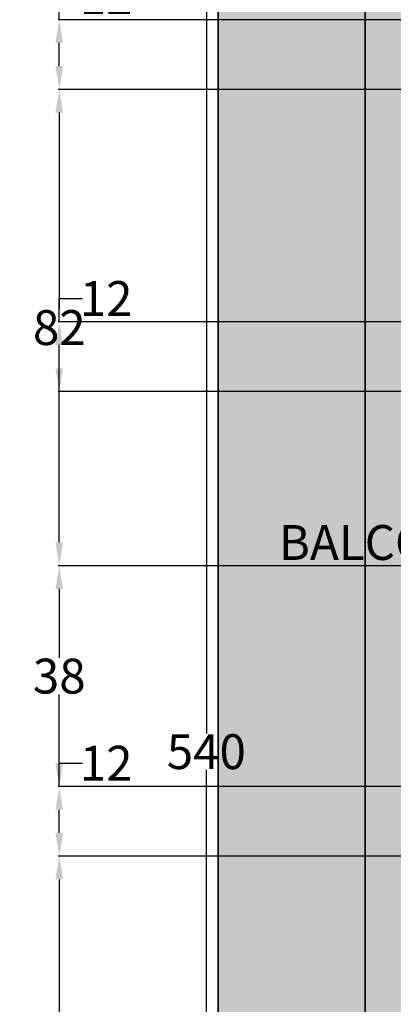
# Model space of a CAD drawing. Units: inches. Extents: x 184 to 649, y 215 to 818.
# Tile 4 of 9: x 189 to 254, y 473 to 643. Entities that reach past the tile are written whole.
import ezdxf

# ---------------------------------------------------------------- set-up
doc = ezdxf.new("R2010")
doc.units = ezdxf.units.IN
doc.header["$MEASUREMENT"] = 0
for name, color, linetype, lineweight in [('A-ANNO-DIMS', 2, 'Continuous', 18), ('A-ELEV', 7, 'Continuous', 35), ('A-ELEV-FILL', 9, 'Continuous', 13)]:
    doc.layers.add(name, color=color, linetype=linetype, lineweight=lineweight)
doc.styles.get("Standard").update_dxf_attribs({"font": 'arial.ttf'})
doc.dimstyles.get("Standard").update_dxf_attribs({"dimtxt": 6, "dimasz": 4, "dimexe": 0.18, "dimexo": 0.0625, "dimgap": 0.09, "dimtad": 0, "dimtih": 1, "dimtoh": 1, "dimdec": 0, "dimzin": 0, "dimdsep": 46, "dimlunit": 3, "dimtxsty": 'Standard', "dimcen": 0.09, "dimadec": 0, "dimazin": 0, "dimtfac": 1, "dimtdec": 0, "dimtofl": 0, "dimtmove": 0, "dimatfit": 3, "dimfxl": 1, "dimtolj": 1, "dimtzin": 0, "dimarcsym": 0})

# ---------------------------------------------------------------- blocks, each defined once
blk = doc.blocks.new('*D7')
at = {"layer": 'A-ANNO-DIMS', "color": 0, "lineweight": -2, "transparency": 16777216}
for p, q in [((291.94, 594.73), (279.22, 594.73)), ((279.4, 590.73), (279.4, 555.92)), ((279.4, 514.73), (279.4, 549.53)), ((291.94, 510.73), (279.22, 510.73))]:
    blk.add_line(p, q, dxfattribs=at)
at = {"layer": 'A-ANNO-DIMS', "color": 0, "transparency": 16777216}
for points in [[(278.73, 590.73), (280.07, 590.73), (279.4, 594.73)], [(278.73, 514.73), (280.07, 514.73), (279.4, 510.73)]]:
    blk.add_solid(points, dxfattribs=at)
at = {"layer": 'Defpoints', "color": 0, "transparency": 16777216}
for p in [(279.4, 594.73), (292, 594.73), (292, 510.73)]:
    blk.add_point(p, dxfattribs=at)
at = {"layer": 'A-ANNO-DIMS', "color": 0, "transparency": 16777216, "insert": (279.4, 552.73), "char_height": 6, "attachment_point": 5}
blk.add_mtext('\\A1;BALCONY DOOR 84 TYP.', dxfattribs=at)
blk = doc.blocks.new('*D10')
at = {"layer": 'A-ANNO-DIMS', "color": 0, "lineweight": -2, "transparency": 16777216}
for p, q in [((248.91, 786.73), (221.44, 786.73)), ((221.62, 782.73), (221.62, 519.88)), ((221.62, 250.73), (221.62, 513.57)), ((248.91, 246.73), (221.44, 246.73))]:
    blk.add_line(p, q, dxfattribs=at)
at = {"layer": 'A-ANNO-DIMS', "color": 0, "transparency": 16777216}
for points in [[(220.96, 782.73), (222.29, 782.73), (221.62, 786.73)], [(220.96, 250.73), (222.29, 250.73), (221.62, 246.73)]]:
    blk.add_solid(points, dxfattribs=at)
at = {"layer": 'Defpoints', "color": 0, "transparency": 16777216}
for p in [(221.62, 786.73), (248.97, 786.73), (248.97, 246.73)]:
    blk.add_point(p, dxfattribs=at)
at = {"layer": 'A-ANNO-DIMS', "color": 0, "transparency": 16777216, "insert": (221.62, 516.73), "char_height": 6, "attachment_point": 5}
blk.add_mtext('\\A1;540', dxfattribs=at)
blk = doc.blocks.new('*D35')
at = {"layer": 'A-ANNO-DIMS', "color": 0, "lineweight": -2, "transparency": 16777216}
for p, q in [((260.91, 498.73), (196.12, 498.73)), ((196.3, 494.73), (196.3, 437.38)), ((196.3, 373.73), (196.3, 431.07)), ((260.91, 369.73), (196.12, 369.73))]:
    blk.add_line(p, q, dxfattribs=at)
at = {"layer": 'A-ANNO-DIMS', "color": 0, "transparency": 16777216}
for points in [[(195.63, 494.73), (196.96, 494.73), (196.3, 498.73)], [(195.63, 373.73), (196.96, 373.73), (196.3, 369.73)]]:
    blk.add_solid(points, dxfattribs=at)
at = {"layer": 'Defpoints', "color": 0, "transparency": 16777216}
for p in [(196.3, 498.73), (260.97, 498.73), (260.97, 369.73)]:
    blk.add_point(p, dxfattribs=at)
at = {"layer": 'A-ANNO-DIMS', "color": 0, "transparency": 16777216, "insert": (196.3, 434.23), "char_height": 6, "attachment_point": 5}
blk.add_mtext('\\A1;129', dxfattribs=at)
blk = doc.blocks.new('*D36')
at = {"layer": 'A-ANNO-DIMS', "color": 0, "lineweight": -2, "transparency": 16777216}
for p, q in [((196.3, 510.73), (196.3, 514.73)), ((196.3, 514.73), (200.3, 514.73)), ((260.91, 510.73), (196.12, 510.73)), ((196.3, 502.73), (196.3, 506.73)), ((260.91, 498.73), (196.12, 498.73))]:
    blk.add_line(p, q, dxfattribs=at)
at = {"layer": 'A-ANNO-DIMS', "color": 0, "transparency": 16777216}
for points in [[(195.63, 506.73), (196.96, 506.73), (196.3, 510.73)], [(195.63, 502.73), (196.96, 502.73), (196.3, 498.73)]]:
    blk.add_solid(points, dxfattribs=at)
at = {"layer": 'Defpoints', "color": 0, "transparency": 16777216}
for p in [(196.3, 510.73), (260.97, 510.73), (260.97, 498.73)]:
    blk.add_point(p, dxfattribs=at)
at = {"layer": 'A-ANNO-DIMS', "color": 0, "transparency": 16777216, "insert": (204.37, 514.73), "char_height": 6, "attachment_point": 5}
blk.add_mtext('\\A1;12', dxfattribs=at)
blk = doc.blocks.new('*D37')
at = {"layer": 'A-ANNO-DIMS', "color": 0, "lineweight": -2, "transparency": 16777216}
for p, q in [((260.91, 548.73), (196.12, 548.73)), ((196.3, 544.73), (196.3, 532.88)), ((196.3, 514.73), (196.3, 526.57)), ((260.91, 510.73), (196.12, 510.73))]:
    blk.add_line(p, q, dxfattribs=at)
at = {"layer": 'A-ANNO-DIMS', "color": 0, "transparency": 16777216}
for points in [[(195.63, 544.73), (196.96, 544.73), (196.3, 548.73)], [(195.63, 514.73), (196.96, 514.73), (196.3, 510.73)]]:
    blk.add_solid(points, dxfattribs=at)
at = {"layer": 'Defpoints', "color": 0, "transparency": 16777216}
for p in [(196.3, 548.73), (260.97, 548.73), (260.97, 510.73)]:
    blk.add_point(p, dxfattribs=at)
at = {"layer": 'A-ANNO-DIMS', "color": 0, "transparency": 16777216, "insert": (196.3, 529.73), "char_height": 6, "attachment_point": 5}
blk.add_mtext('\\A1;38', dxfattribs=at)
blk = doc.blocks.new('*D38')
at = {"layer": 'A-ANNO-DIMS', "color": 0, "lineweight": -2, "transparency": 16777216}
for p, q in [((260.91, 630.73), (196.12, 630.73)), ((196.3, 626.73), (196.3, 592.88)), ((196.3, 552.73), (196.3, 586.57)), ((260.91, 548.73), (196.12, 548.73))]:
    blk.add_line(p, q, dxfattribs=at)
at = {"layer": 'A-ANNO-DIMS', "color": 0, "transparency": 16777216}
for points in [[(195.63, 626.73), (196.96, 626.73), (196.3, 630.73)], [(195.63, 552.73), (196.96, 552.73), (196.3, 548.73)]]:
    blk.add_solid(points, dxfattribs=at)
at = {"layer": 'Defpoints', "color": 0, "transparency": 16777216}
for p in [(196.3, 630.73), (260.97, 630.73), (260.97, 548.73)]:
    blk.add_point(p, dxfattribs=at)
at = {"layer": 'A-ANNO-DIMS', "color": 0, "transparency": 16777216, "insert": (196.3, 589.73), "char_height": 6, "attachment_point": 5}
blk.add_mtext('\\A1;82', dxfattribs=at)
blk = doc.blocks.new('*D39')
at = {"layer": 'A-ANNO-DIMS', "color": 0, "lineweight": -2, "transparency": 16777216}
for p, q in [((196.3, 642.73), (196.3, 646.73)), ((196.3, 646.73), (200.3, 646.73)), ((260.91, 642.73), (196.12, 642.73)), ((196.3, 634.73), (196.3, 638.73)), ((260.91, 630.73), (196.12, 630.73))]:
    blk.add_line(p, q, dxfattribs=at)
at = {"layer": 'A-ANNO-DIMS', "color": 0, "transparency": 16777216}
for points in [[(195.63, 638.73), (196.96, 638.73), (196.3, 642.73)], [(195.63, 634.73), (196.96, 634.73), (196.3, 630.73)]]:
    blk.add_solid(points, dxfattribs=at)
at = {"layer": 'Defpoints', "color": 0, "transparency": 16777216}
for p in [(196.3, 642.73), (260.97, 642.73), (260.97, 630.73)]:
    blk.add_point(p, dxfattribs=at)
at = {"layer": 'A-ANNO-DIMS', "color": 0, "transparency": 16777216, "insert": (204.37, 646.73), "char_height": 6, "attachment_point": 5}
blk.add_mtext('\\A1;12', dxfattribs=at)
blk = doc.blocks.new('*D61')
at = {"layer": 'A-ANNO-DIMS', "color": 0, "lineweight": -2, "transparency": 16777216}
for p, q in [((196.3, 590.73), (196.3, 594.73)), ((196.3, 594.73), (200.3, 594.73)), ((295.94, 590.73), (196.12, 590.73)), ((196.3, 582.73), (196.3, 586.73)), ((295.94, 578.73), (196.12, 578.73))]:
    blk.add_line(p, q, dxfattribs=at)
at = {"layer": 'A-ANNO-DIMS', "color": 0, "transparency": 16777216}
for points in [[(195.63, 586.73), (196.96, 586.73), (196.3, 590.73)], [(195.63, 582.73), (196.96, 582.73), (196.3, 578.73)]]:
    blk.add_solid(points, dxfattribs=at)
at = {"layer": 'Defpoints', "color": 0, "transparency": 16777216}
for p in [(196.3, 590.73), (296, 590.73), (296, 578.73)]:
    blk.add_point(p, dxfattribs=at)
at = {"layer": 'A-ANNO-DIMS', "color": 0, "transparency": 16777216, "insert": (204.37, 594.73), "char_height": 6, "attachment_point": 5}
blk.add_mtext('\\A1;12', dxfattribs=at)

msp = doc.modelspace()

# ---------------------------------------------------------------- hatches: boundary and pattern name
at = {"layer": 'A-ELEV-FILL'}
h = msp.add_hatch(color=256, dxfattribs=at)
h.dxf.hatch_style = 1
h.paths.add_polyline_path([(248.9726, 786.7265), (223.6471, 761.141), (223.6471, 257.141), (248.9726, 246.7265)])
h = msp.add_hatch(color=256, dxfattribs=at)
h.dxf.hatch_style = 1
h.paths.add_polyline_path([(452.9726, 369.7265), (248.9726, 369.7265), (248.9726, 246.7265), (275.9726, 246.7265), (275.9726, 328.7265), (437.9726, 328.7265), (437.9726, 246.7265), (446.6666, 246.7265), (452.9726, 282.7265)])
h.paths.add_polyline_path([(275.9726, 340.7265), (275.9726, 354.7265), (437.9726, 354.7265), (437.9726, 340.7265)], flags=16)
h.paths.add_polyline_path([(452.9726, 510.7265), (260.9726, 510.7265), (260.9726, 642.7265), (260.9726, 699.7265), (367.0226, 699.7265), (373.9381, 706.7265), (260.9726, 706.7265), (260.9726, 715.7265), (382.8295, 715.7265), (389.745, 722.7265), (260.9726, 722.7265), (260.9726, 731.7265), (398.6364, 731.7265), (405.5519, 738.7265), (260.9726, 738.7265), (260.9726, 747.7265), (414.4433, 747.7265), (421.3588, 754.7265), (260.9726, 754.7265), (260.9726, 763.7265), (430.2502, 763.7265), (437.1657, 770.7265), (260.9726, 770.7265), (260.9726, 779.7265), (446.057, 779.7265), (452.9726, 786.7265), (248.9726, 786.7265), (248.9726, 369.7265), (260.9726, 369.7265), (260.9726, 498.7265), (452.9726, 498.7265)])

# ---------------------------------------------------------------- linework, layer by layer
at = {"layer": 'A-ELEV'}
for p, q in [((248.9726, 786.7265), (248.9726, 246.7265)), ((223.6471, 761.141), (223.6471, 257.141))]:
    msp.add_line(p, q, dxfattribs=at)

# ---------------------------------------------------------------- dimensions: what is measured, and where the dimension line sits
at = {"layer": 'A-ANNO-DIMS'}
for base, p1, p2, picture, middle in [((221.6226, 786.7265), (248.9726, 246.7265), (248.9726, 786.7265), '*D10', (221.6226, 516.7265)), ((196.2971, 642.7265), (260.9726, 630.7265), (260.9726, 642.7265), '*D39', (204.3714, 646.7265)), ((196.2971, 630.7265), (260.9726, 548.7265), (260.9726, 630.7265), '*D38', (196.2971, 589.7265)), ((196.2971, 590.7265), (295.9998, 578.7265), (295.9998, 590.7265), '*D61', (204.3714, 594.7265)), ((196.2971, 548.7265), (260.9726, 510.7265), (260.9726, 548.7265), '*D37', (196.2971, 529.7265)), ((196.2971, 510.7265), (260.9726, 498.7265), (260.9726, 510.7265), '*D36', (204.3714, 514.7265)), ((196.2971, 498.7265), (260.9726, 369.7265), (260.9726, 498.7265), '*D35', (196.2971, 434.2265))]:
    dim = msp.add_linear_dim(base=base, p1=p1, p2=p2, angle=90, dimstyle='Standard', override={"dimdec": 0, "dimlfac": 1, "dimrnd": 0, "dimzin": 0, "dimdsep": 46, "dimlunit": 2}, dxfattribs=at)
    dim.commit()
    dim.dimension.update_dxf_attribs({"geometry": picture, "text_midpoint": middle})
dim = msp.add_linear_dim(base=(279.3998, 594.7265), p1=(291.9998, 510.7265), p2=(291.9998, 594.7265), angle=90, text='BALCONY DOOR <> TYP.', dimstyle='Standard', override={"dimdec": 0, "dimrnd": 0, "dimzin": 0, "dimlunit": 2}, dxfattribs=at)
dim.commit()
dim.dimension.update_dxf_attribs({"geometry": '*D7', "text_midpoint": (279.3998, 552.7265)})

doc.saveas('drawing.dxf')
